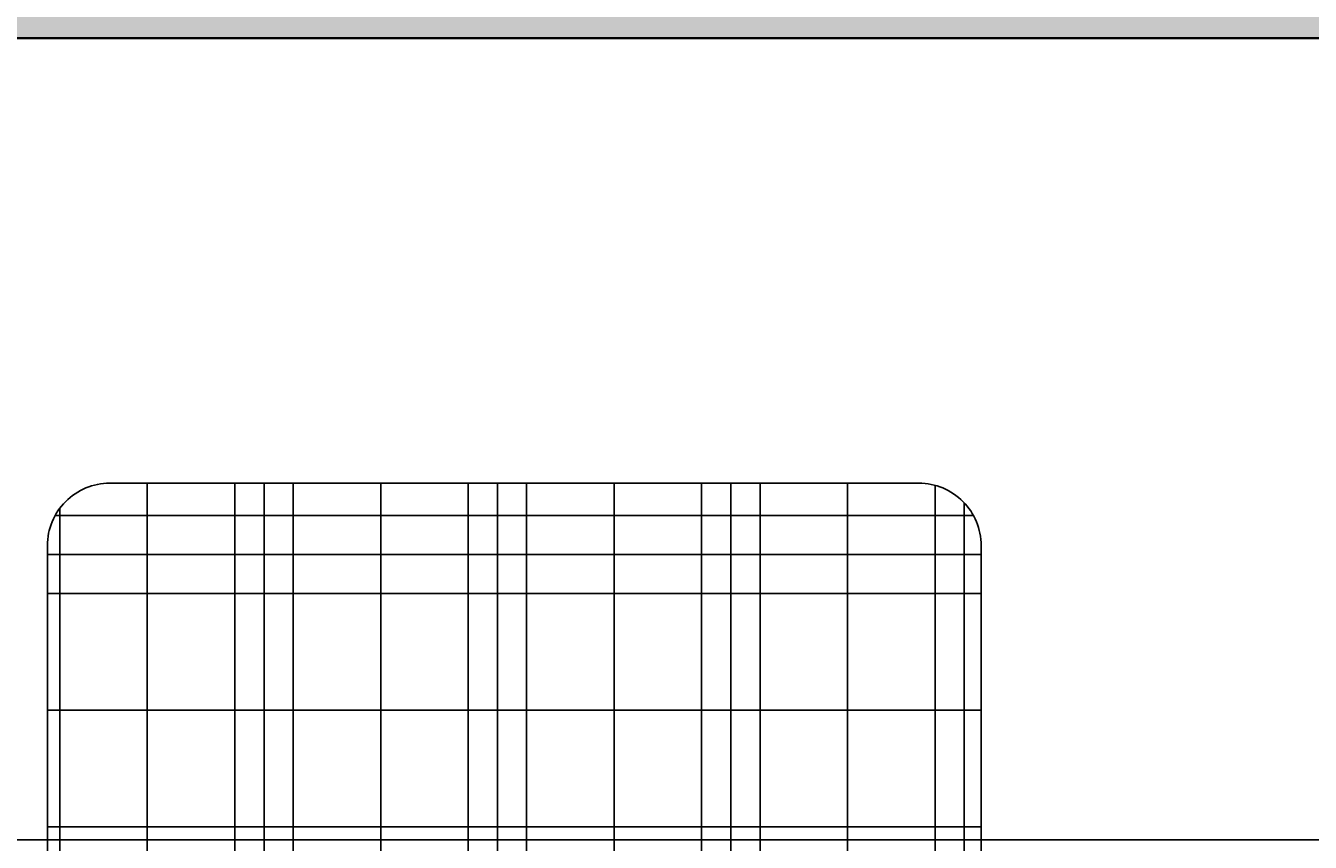
# Model space of a CAD drawing. Units: millimetres. Extents: x 2817 to 5038, y 1110 to 3565.
# Tile 7 of 21: x 2870 to 2946, y 1323 to 1371. Entities that reach past the tile are written whole.
import ezdxf

# ---------------------------------------------------------------- set-up
doc = ezdxf.new("R2010")
doc.units = ezdxf.units.MM
for name, color, linetype, lineweight in [('A-ANNO-DIMS', 2, 'Continuous', 18), ('A-WALL', 7, 'Continuous', 35), ('FURNITURE', 219, 'Continuous', 18)]:
    doc.layers.add(name, color=color, linetype=linetype, lineweight=lineweight)
doc.layers.add('A-WALL-PATT', color=51, linetype='Continuous', lineweight=13, true_color=0xf7f281)
doc.layers.add('BLOCK', color=6, linetype='Continuous')
doc.styles.get("Standard").update_dxf_attribs({"font": 'arial.ttf'})
doc.dimstyles.get("Standard").update_dxf_attribs({"dimtxt": 0.18, "dimasz": 0.18, "dimexe": 0.18, "dimexo": 0.0625, "dimgap": 0.09, "dimtad": 0, "dimtih": 1, "dimtoh": 1, "dimdec": 4, "dimzin": 0, "dimdsep": 46, "dimtxsty": 'Standard', "dimcen": 0.09, "dimadec": 0, "dimazin": 0, "dimtfac": 1, "dimtdec": 4, "dimtofl": 0, "dimtmove": 0, "dimatfit": 3, "dimfxl": 1, "dimtolj": 1, "dimtzin": 0, "dimarcsym": 0})

# ---------------------------------------------------------------- blocks, each defined once
blk = doc.blocks.new('*X7')
at = {"color": 0}
for p, q in [((276.598, 451.25), (280.51, 451.25)), ((275.455, 450.625), (280.51, 450.625)), ((274.411, 450), (280.51, 450)), ((265.51, 448.125), (267.634, 448.125)), ((271.723, 448.125), (280.51, 448.125)), ((265.51, 446.25), (268.465, 446.25)), ((269.519, 446.25), (280.51, 446.25)), ((265.51, 445.625), (268.531, 445.625)), ((268.866, 445.625), (280.51, 445.625)), ((265.51, 445), (280.51, 445)), ((265.51, 443.125), (280.51, 443.125)), ((265.51, 441.25), (280.51, 441.25)), ((265.51, 440.625), (280.51, 440.625)), ((265.634, 440), (280.386, 440))]:
    blk.add_line(p, q, dxfattribs=at)
blk = doc.blocks.new('*X8')
at = {"color": 0}
for p, q in [((280.312, 439.886), (280.312, 452.896)), ((278.906, 439.482), (278.906, 452.338)), ((277.5, 439.482), (277.5, 451.702)), ((277.031, 439.482), (277.031, 451.471)), ((276.562, 439.482), (276.562, 451.231)), ((275.156, 439.482), (275.156, 450.451)), ((265.781, 439.797), (265.781, 449.511)), ((273.75, 439.482), (273.75, 449.576)), ((266.25, 439.517), (266.25, 449.296)), ((273.281, 439.482), (273.281, 449.261)), ((272.812, 439.482), (272.812, 448.934)), ((267.656, 439.482), (267.656, 448.095)), ((271.406, 439.482), (271.406, 447.876)), ((270, 439.482), (270, 446.689)), ((269.531, 439.482), (269.531, 446.262)), ((269.062, 439.482), (269.062, 445.817))]:
    blk.add_line(p, q, dxfattribs=at)
blk = doc.blocks.new('A$C52E67D0D')
at = {"layer": 'BLOCK'}
blk.add_lwpolyline([(1901, 0), (601, 0, -0.414214), (501, 100), (501, 1700, -0.414214), (601, 1800), (1901, 1800, -0.414214), (2001, 1700), (2001, 100, -0.414214)], format="xyb", close=True, dxfattribs=at)
at = {"layer": 'BLOCK', "xscale": 100, "yscale": 100, "zscale": 100}
for name in ['*X8', '*X7']:
    blk.add_blockref(name, (-26050, -43948.2), dxfattribs=at)
blk = doc.blocks.new('*D47')
at = {"layer": 'A-ANNO-DIMS', "color": 0, "lineweight": -2, "transparency": 16777216}
for p, q in [((3052.177, 1370.436), (2817.308, 1370.436)), ((2817.488, 1370.256), (2817.488, 1346.949)), ((2817.488, 1323.278), (2817.488, 1346.585)), ((3052.075, 1323.098), (2817.308, 1323.098))]:
    blk.add_line(p, q, dxfattribs=at)
for points in [[(2817.458, 1370.256), (2817.518, 1370.256), (2817.488, 1370.436)], [(2817.458, 1323.278), (2817.518, 1323.278), (2817.488, 1323.098)]]:
    blk.add_solid(points, dxfattribs=at)
at = {"layer": 'Defpoints', "color": 0, "lineweight": -2, "transparency": 16777216}
for p in [(2817.488, 1370.436), (3052.239, 1370.436), (3052.138, 1323.098)]:
    blk.add_point(p, dxfattribs=at)
at = {"layer": 'A-ANNO-DIMS', "color": 0, "transparency": 16777216, "insert": (2817.488, 1346.767), "char_height": 0.18, "attachment_point": 5}
blk.add_mtext('\\A1;47.34', dxfattribs=at)

msp = doc.modelspace()

# ---------------------------------------------------------------- hatches: boundary and pattern name
at = {"layer": 'A-WALL-PATT'}
h = msp.add_hatch(color=256, dxfattribs=at)
h.dxf.hatch_style = 1
h.paths.add_polyline_path([(3186.7393, 1614.4357), (2841.7393, 1614.4357), (2841.7393, 1568.614), (2850.7393, 1568.7609), (2850.7393, 1605.4357), (2982.7393, 1605.4357), (2991.7393, 1605.4357), (3052.2393, 1605.4357), (3052.2393, 1573.7835), (3061.2393, 1573.7835), (3061.2393, 1605.4357), (3182.2393, 1605.4357), (3182.2393, 1143.4357), (3181.2393, 1143.4357), (3181.2393, 1134.4357), (3186.7393, 1134.4357)])
h.paths.add_polyline_path([(3061.2393, 1143.4357), (3061.2393, 1147.4357), (3052.2393, 1147.4357), (3052.2393, 1143.4357), (2850.7393, 1143.4357), (2850.7393, 1145.2996), (2841.7393, 1145.2996), (2841.7393, 1134.4357), (3061.2393, 1134.4357)], flags=17)
h.paths.add_polyline_path([(2850.7393, 1265.4357), (2946.7393, 1265.4357), (2946.7393, 1270.8357), (2946.7393, 1274.4357), (2850.7393, 1274.4357), (2850.7381, 1274.4357), (2850.7381, 1274.2564), (2841.7393, 1274.2564), (2841.7393, 1193.1527), (2850.7393, 1193.2996)], flags=17)
h.paths.add_polyline_path([(3061.2393, 1299.098), (3052.2393, 1299.098), (3052.2393, 1274.4357), (2991.7393, 1274.4357), (2991.7393, 1340.4357), (2982.7393, 1340.4357), (2982.7393, 1274.4357), (2982.7393, 1265.4357), (3052.2393, 1265.4357), (3052.2393, 1259.143), (3061.2393, 1259.2899)], flags=17)
h.paths.add_polyline_path([(3061.2393, 1383.4357), (3052.2393, 1383.4357), (3052.2393, 1379.4357), (2931.7393, 1379.4357), (2922.7393, 1379.4357), (2850.7393, 1379.4357), (2850.7381, 1379.4357), (2850.7381, 1379.3646), (2841.7393, 1379.3646), (2841.7393, 1322.1095), (2850.7393, 1322.2564), (2850.7393, 1370.4357), (2982.7393, 1370.4357), (2987.2393, 1370.4357), (3017.2393, 1370.4357), (3052.2393, 1370.4357), (3052.2393, 1323.098), (3061.2393, 1323.098)], flags=17)

# ---------------------------------------------------------------- linework, layer by layer
at = {"layer": 'A-WALL'}
msp.add_line((2850.7393, 1370.4357), (2982.7393, 1370.4357), dxfattribs=at)

# ---------------------------------------------------------------- block references
at = {"layer": 'FURNITURE', "xscale": 0.0367705835331598, "yscale": 0.0367705835331598, "zscale": 0.0367705835331598, "rotation": 180}
msp.add_blockref('A$C52E67D0D', (2944.6948, 1344.1495), dxfattribs=at)

# ---------------------------------------------------------------- dimensions: what is measured, and where the dimension line sits
at = {"layer": 'A-ANNO-DIMS'}
dim = msp.add_linear_dim(base=(2817.4881, 1370.4357), p1=(3052.1378, 1323.098), p2=(3052.2393, 1370.4357), angle=90, dimstyle='Standard', override={"dimdec": 2, "dimlfac": 1, "dimrnd": 0, "dimzin": 0, "dimdsep": 46, "dimlunit": 2}, dxfattribs=at)
dim.commit()
dim.dimension.update_dxf_attribs({"geometry": '*D47', "text_midpoint": (2817.4881, 1346.7669)})

doc.saveas('drawing.dxf')
